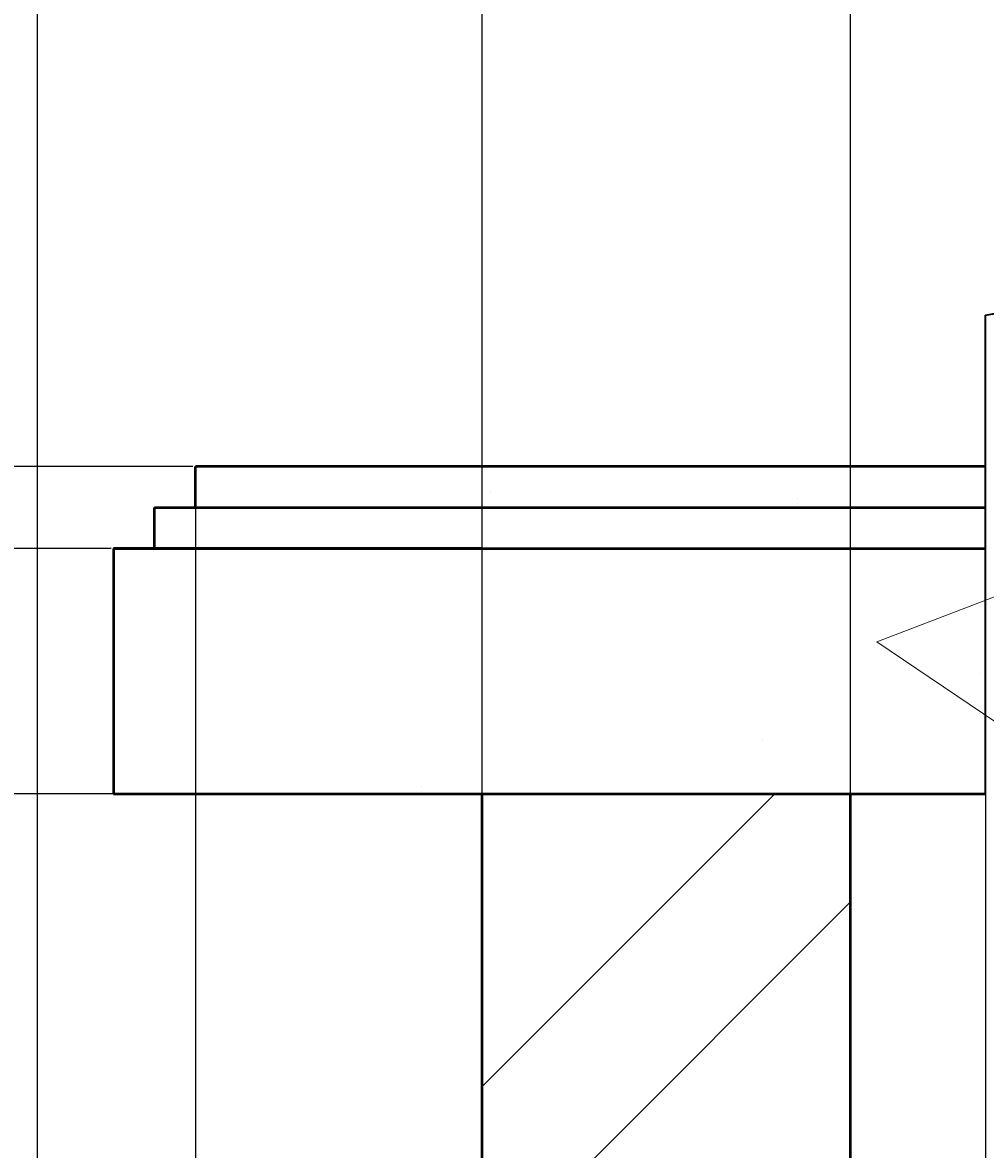
# Model space of a CAD drawing. Units: inches. Extents: x 2812 to 3051, y 1398 to 1659.
# Tile 8 of 65: x 2824 to 2848, y 1473 to 1501. Entities that reach past the tile are written whole.
import ezdxf

# ---------------------------------------------------------------- set-up
doc = ezdxf.new("R2010")
doc.units = ezdxf.units.IN
for name, color, linetype, lineweight in [('A-ANNO-DIMS', 2, 'Continuous', 18), ('P-SANR-PIPE', 4, 'Continuous', 35), ('S-CONC', 7, 'Continuous', 50), ('S-CONC-PATT', 8, 'Continuous', 18)]:
    doc.layers.add(name, color=color, linetype=linetype, lineweight=lineweight)
doc.styles.get("Standard").update_dxf_attribs({"font": 'arial.ttf'})
doc.dimstyles.get("Standard").update_dxf_attribs({"dimtxt": 0.18, "dimasz": 0.18, "dimexe": 0.18, "dimexo": 0.0625, "dimgap": 0.09, "dimtad": 0, "dimtih": 1, "dimtoh": 1, "dimdec": 4, "dimzin": 0, "dimdsep": 46, "dimtxsty": 'Standard', "dimcen": 0.09, "dimadec": 0, "dimazin": 0, "dimtfac": 1, "dimtdec": 4, "dimtofl": 0, "dimtmove": 0, "dimatfit": 3, "dimfxl": 1, "dimtolj": 1, "dimtzin": 0, "dimarcsym": 0})

# ---------------------------------------------------------------- blocks, each defined once
blk = doc.blocks.new('*D27')
at = {"layer": 'A-ANNO-DIMS', "color": 0, "lineweight": -2, "transparency": 16777216}
for p, q in [((2824.521, 1594.167), (2824.521, 1397.505)), ((2835.385, 1550.757), (2835.385, 1397.505)), ((2824.701, 1397.685), (2829.498, 1397.685)), ((2835.205, 1397.685), (2830.408, 1397.685))]:
    blk.add_line(p, q, dxfattribs=at)
at = {"layer": 'A-ANNO-DIMS', "color": 0, "transparency": 16777216}
for points in [[(2824.701, 1397.715), (2824.701, 1397.655), (2824.521, 1397.685)], [(2835.205, 1397.715), (2835.205, 1397.655), (2835.385, 1397.685)]]:
    blk.add_solid(points, dxfattribs=at)
at = {"layer": 'Defpoints', "color": 0, "transparency": 16777216}
for p in [(2824.521, 1594.23), (2835.385, 1550.82), (2835.385, 1397.685)]:
    blk.add_point(p, dxfattribs=at)
at = {"layer": 'A-ANNO-DIMS', "color": 0, "transparency": 16777216, "insert": (2829.953, 1397.685), "char_height": 0.18, "attachment_point": 5}
blk.add_mtext('\\A1;10.863', dxfattribs=at)
blk = doc.blocks.new('*D28')
at = {"layer": 'A-ANNO-DIMS', "color": 0, "lineweight": -2, "transparency": 16777216}
for p, q in [((2851.646, 1598.667), (2851.646, 1397.505)), ((2844.385, 1559.757), (2844.385, 1397.505)), ((2844.565, 1397.685), (2847.64, 1397.685)), ((2851.466, 1397.685), (2848.391, 1397.685))]:
    blk.add_line(p, q, dxfattribs=at)
at = {"layer": 'A-ANNO-DIMS', "color": 0, "transparency": 16777216}
for points in [[(2844.565, 1397.715), (2844.565, 1397.655), (2844.385, 1397.685)], [(2851.466, 1397.715), (2851.466, 1397.655), (2851.646, 1397.685)]]:
    blk.add_solid(points, dxfattribs=at)
at = {"layer": 'Defpoints', "color": 0, "transparency": 16777216}
for p in [(2851.646, 1598.73), (2844.385, 1559.82), (2851.646, 1397.685)]:
    blk.add_point(p, dxfattribs=at)
at = {"layer": 'A-ANNO-DIMS', "color": 0, "transparency": 16777216, "insert": (2848.016, 1397.685), "char_height": 0.18, "attachment_point": 5}
blk.add_mtext('\\A1;7.261', dxfattribs=at)
blk = doc.blocks.new('*D41')
at = {"layer": 'A-ANNO-DIMS', "color": 0, "lineweight": -2, "transparency": 16777216}
for p, q in [((2828.385, 1489.973), (2828.385, 1397.505)), ((2826.385, 1409.973), (2826.385, 1397.505)), ((2826.565, 1397.685), (2827.235, 1397.685)), ((2828.205, 1397.685), (2827.535, 1397.685))]:
    blk.add_line(p, q, dxfattribs=at)
at = {"layer": 'A-ANNO-DIMS', "color": 0, "transparency": 16777216}
for points in [[(2826.565, 1397.715), (2826.565, 1397.655), (2826.385, 1397.685)], [(2828.205, 1397.715), (2828.205, 1397.655), (2828.385, 1397.685)]]:
    blk.add_solid(points, dxfattribs=at)
at = {"layer": 'Defpoints', "color": 0, "transparency": 16777216}
for p in [(2828.385, 1490.035), (2826.385, 1410.035), (2828.385, 1397.685)]:
    blk.add_point(p, dxfattribs=at)
at = {"layer": 'A-ANNO-DIMS', "color": 0, "transparency": 16777216, "insert": (2827.385, 1397.685), "char_height": 0.18, "attachment_point": 5}
blk.add_mtext('\\A1;2', dxfattribs=at)
blk = doc.blocks.new('*D42')
at = {"layer": 'A-ANNO-DIMS', "color": 0, "lineweight": -2, "transparency": 16777216}
for p, q in [((2828.385, 1489.973), (2828.385, 1397.505)), ((2847.686, 1487.973), (2847.686, 1397.505)), ((2828.565, 1397.685), (2837.72, 1397.685)), ((2847.506, 1397.685), (2838.351, 1397.685))]:
    blk.add_line(p, q, dxfattribs=at)
at = {"layer": 'A-ANNO-DIMS', "color": 0, "transparency": 16777216}
for points in [[(2828.565, 1397.715), (2828.565, 1397.655), (2828.385, 1397.685)], [(2847.506, 1397.715), (2847.506, 1397.655), (2847.686, 1397.685)]]:
    blk.add_solid(points, dxfattribs=at)
at = {"layer": 'Defpoints', "color": 0, "transparency": 16777216}
for p in [(2828.385, 1490.035), (2847.686, 1488.035), (2847.686, 1397.685)]:
    blk.add_point(p, dxfattribs=at)
at = {"layer": 'A-ANNO-DIMS', "color": 0, "transparency": 16777216, "insert": (2838.036, 1397.685), "char_height": 0.18, "attachment_point": 5}
blk.add_mtext('\\A1;19.3', dxfattribs=at)
blk = doc.blocks.new('*D51')
at = {"layer": 'A-ANNO-DIMS', "color": 0, "lineweight": -2, "transparency": 16777216}
for p, q in [((2835.322, 1482.035), (2811.806, 1482.035)), ((2811.986, 1481.855), (2811.986, 1472.351)), ((2811.986, 1462.483), (2811.986, 1471.987)), ((2835.322, 1462.303), (2811.806, 1462.303))]:
    blk.add_line(p, q, dxfattribs=at)
at = {"layer": 'A-ANNO-DIMS', "color": 0, "transparency": 16777216}
for points in [[(2811.956, 1481.855), (2812.016, 1481.855), (2811.986, 1482.035)], [(2811.956, 1462.483), (2812.016, 1462.483), (2811.986, 1462.303)]]:
    blk.add_solid(points, dxfattribs=at)
at = {"layer": 'Defpoints', "color": 0, "transparency": 16777216}
for p in [(2811.986, 1482.035), (2835.385, 1482.035), (2835.385, 1462.303)]:
    blk.add_point(p, dxfattribs=at)
at = {"layer": 'A-ANNO-DIMS', "color": 0, "transparency": 16777216, "insert": (2811.986, 1472.169), "char_height": 0.18, "attachment_point": 5}
blk.add_mtext('\\A1;19.733', dxfattribs=at)
blk = doc.blocks.new('*D52')
at = {"layer": 'A-ANNO-DIMS', "color": 0, "lineweight": -2, "transparency": 16777216}
for p, q in [((2826.322, 1488.035), (2811.806, 1488.035)), ((2811.986, 1487.855), (2811.986, 1485.217)), ((2811.986, 1482.215), (2811.986, 1484.853)), ((2826.322, 1482.035), (2811.806, 1482.035))]:
    blk.add_line(p, q, dxfattribs=at)
at = {"layer": 'A-ANNO-DIMS', "color": 0, "transparency": 16777216}
for points in [[(2811.956, 1487.855), (2812.016, 1487.855), (2811.986, 1488.035)], [(2811.956, 1482.215), (2812.016, 1482.215), (2811.986, 1482.035)]]:
    blk.add_solid(points, dxfattribs=at)
at = {"layer": 'Defpoints', "color": 0, "transparency": 16777216}
for p in [(2811.986, 1488.035), (2826.385, 1488.035), (2826.385, 1482.035)]:
    blk.add_point(p, dxfattribs=at)
at = {"layer": 'A-ANNO-DIMS', "color": 0, "transparency": 16777216, "insert": (2811.986, 1485.035), "char_height": 0.18, "attachment_point": 5}
blk.add_mtext('\\A1;6', dxfattribs=at)
blk = doc.blocks.new('*D53')
at = {"layer": 'A-ANNO-DIMS', "color": 0, "lineweight": -2, "transparency": 16777216}
for p, q in [((2828.322, 1490.035), (2811.806, 1490.035)), ((2811.986, 1489.855), (2811.986, 1489.216)), ((2811.986, 1488.215), (2811.986, 1488.855)), ((2826.322, 1488.035), (2811.806, 1488.035))]:
    blk.add_line(p, q, dxfattribs=at)
at = {"layer": 'A-ANNO-DIMS', "color": 0, "transparency": 16777216}
for points in [[(2811.956, 1489.855), (2812.016, 1489.855), (2811.986, 1490.035)], [(2811.956, 1488.215), (2812.016, 1488.215), (2811.986, 1488.035)]]:
    blk.add_solid(points, dxfattribs=at)
at = {"layer": 'Defpoints', "color": 0, "transparency": 16777216}
for p in [(2811.986, 1490.035), (2828.385, 1490.035), (2826.385, 1488.035)]:
    blk.add_point(p, dxfattribs=at)
at = {"layer": 'A-ANNO-DIMS', "color": 0, "transparency": 16777216, "insert": (2811.986, 1489.035), "char_height": 0.18, "attachment_point": 5}
blk.add_mtext('\\A1;2', dxfattribs=at)

msp = doc.modelspace()

# ---------------------------------------------------------------- hatches: boundary and pattern name
at = {"layer": 'S-CONC-PATT'}
h = msp.add_hatch(dxfattribs=at)
h.set_pattern_fill('ANSI32', color=256)
h.paths.add_polyline_path([(3027.3849, 1646.82), (2835.3849, 1646.82), (2835.3849, 1603.2296), (2844.3849, 1603.2296), (2844.3849, 1637.82), (3018.3849, 1637.82), (3018.3849, 1602.5441), (3027.3849, 1602.5441)])
h.paths.add_polyline_path([(2844.3849, 1594.2296), (2835.3849, 1594.2296), (2835.3849, 1550.82), (3027.3849, 1550.82), (3027.3849, 1593.5441), (3018.3849, 1593.5441), (3018.3849, 1559.82), (2844.3849, 1559.82)])
h.paths.add_polyline_path([(2844.3849, 1482.0354), (2835.3849, 1482.0354), (2835.3849, 1463.4959), (2844.3849, 1463.4959)])
h.paths.add_polyline_path([(2844.3849, 1461.4959), (2835.3849, 1461.4959), (2835.3849, 1416.0354), (2844.3849, 1416.0354)])
h.paths.add_polyline_path([(3027.3849, 1482.0354), (3018.3849, 1482.0354), (3018.3849, 1463.2854), (3027.3849, 1463.2854)])
h.paths.add_polyline_path([(3027.3849, 1461.2854), (3018.3849, 1461.2854), (3018.3849, 1416.0354), (3027.3849, 1416.0354)])
h.paths.add_polyline_path([(2961.3849, 1448.4738), (2952.3849, 1448.4738), (2952.3849, 1416.0354), (2961.3849, 1416.0354)])
h.paths.add_polyline_path([(2961.3849, 1462.3026), (2952.3849, 1462.3026), (2952.3849, 1450.4738), (2961.3849, 1450.4738)])
h.paths.add_polyline_path([(2961.3849, 1472.0354), (2952.3849, 1472.0354), (2952.3849, 1462.3026), (2961.3849, 1462.3026)])
h = msp.add_hatch(dxfattribs=at)
h.set_pattern_fill('AR-SAND', color=256, scale=0.3)
h.paths.add_polyline_path([(3036.3849, 1416.0354), (3027.3849, 1416.0354), (2826.3849, 1416.0354), (2826.3849, 1410.0354), (2835.3849, 1410.0354), (3036.3849, 1410.0354)])
h.paths.add_polyline_path([(2970.3849, 1488.0354), (2969.3849, 1488.0354), (2941.3849, 1488.0354), (2941.3849, 1482.0354), (2970.3849, 1482.0354)])
h.paths.add_polyline_path([(3036.3849, 1488.0354), (3035.3849, 1488.0354), (3006.3849, 1488.0354), (3006.3849, 1482.0354), (3027.3849, 1482.0354), (3036.3849, 1482.0354)])
h.paths.add_polyline_path([(3034.3849, 1490.0354), (3008.3849, 1490.0354), (3008.3849, 1489.0354), (3034.3849, 1489.0354)])
h.paths.add_polyline_path([(3035.3849, 1489.0354), (3034.3849, 1489.0354), (3007.3849, 1489.0354), (3007.3849, 1488.0354), (3035.3849, 1488.0354)])
h.paths.add_polyline_path([(2968.3849, 1490.0354), (2943.3849, 1490.0354), (2943.3849, 1489.0354), (2968.3849, 1489.0354)])
h.paths.add_polyline_path([(2969.3849, 1489.0354), (2968.3849, 1489.0354), (2942.3849, 1489.0354), (2942.3849, 1488.0354), (2969.3849, 1488.0354)])
h.paths.add_polyline_path([(2896.3849, 1488.0354), (2826.3849, 1488.0354), (2826.3849, 1482.0354), (2896.3849, 1482.0354)])
h.paths.add_polyline_path([(2895.3849, 1489.0354), (2894.3849, 1489.0354), (2827.3849, 1489.0354), (2827.3849, 1488.0354), (2895.3849, 1488.0354)])
h.paths.add_polyline_path([(2894.3849, 1490.0354), (2828.3849, 1490.0354), (2828.3849, 1489.0354), (2894.3849, 1489.0354)])
h = msp.add_hatch(dxfattribs=at)
h.set_pattern_fill('AR-CONC', color=256, scale=0.3)
h.paths.add_polyline_path([(2896.3849, 1488.0354), (2826.3849, 1488.0354), (2826.3849, 1482.0354), (2896.3849, 1482.0354)])
h.paths.add_polyline_path([(2970.3849, 1488.0354), (2941.3849, 1488.0354), (2941.3849, 1482.0354), (2970.3849, 1482.0354)])
h.paths.add_polyline_path([(2968.3849, 1490.0354), (2943.3849, 1490.0354), (2943.3849, 1489.0354), (2968.3849, 1489.0354)])
h.paths.add_polyline_path([(2969.3849, 1489.0354), (2968.3849, 1489.0354), (2943.3849, 1489.0354), (2942.3849, 1489.0354), (2942.3849, 1488.0354), (2969.3849, 1488.0354)])
h.paths.add_polyline_path([(3036.3849, 1488.0354), (3035.3849, 1488.0354), (3006.3849, 1488.0354), (3006.3849, 1482.0354), (3027.3849, 1482.0354), (3036.3849, 1482.0354)])
h.paths.add_polyline_path([(3035.3849, 1489.0354), (3034.3849, 1489.0354), (3007.3849, 1489.0354), (3007.3849, 1488.0354), (3035.3849, 1488.0354)])
h.paths.add_polyline_path([(3034.3849, 1490.0354), (3008.3849, 1490.0354), (3008.3849, 1489.0354), (3034.3849, 1489.0354)])
h.paths.add_polyline_path([(2895.3849, 1489.0354), (2894.3849, 1489.0354), (2827.3849, 1489.0354), (2827.3849, 1488.0354), (2895.3849, 1488.0354)])
h.paths.add_polyline_path([(2894.3849, 1490.0354), (2828.3849, 1490.0354), (2828.3849, 1489.0354), (2894.3849, 1489.0354)])

# ---------------------------------------------------------------- linework, layer by layer
at = {"layer": 'P-SANR-PIPE'}
msp.add_line((2847.6863, 1482.0354), (2847.6863, 1493.7383), dxfattribs=at)
msp.add_open_spline([(2847.6863, 1493.7383), (2848.165, 1493.8196), (2849.1224, 1493.9821), (2850.4598, 1493.1692), (2850.7485, 1493.7383)], degree=3, dxfattribs=at)
at = {"layer": 'S-CONC'}
for p, q in [((2828.3849, 1489.0354), (2828.3849, 1490.0354)), ((2847.6863, 1490.0354), (2828.3849, 1490.0354)), ((2827.3849, 1489.0354), (2847.6863, 1489.0354)), ((2827.3849, 1488.0354), (2827.3849, 1489.0354)), ((2827.3849, 1489.0354), (2828.3849, 1489.0354)), ((2826.3849, 1488.0354), (2847.6863, 1488.0354)), ((2835.3849, 1488.0354), (2826.3849, 1488.0354)), ((2826.3849, 1488.0354), (2826.3849, 1482.0354)), ((2826.3849, 1488.0354), (2827.3849, 1488.0354)), ((2826.3849, 1482.0354), (2847.6863, 1482.0354)), ((2835.3849, 1482.0354), (2835.3849, 1416.0354)), ((2835.3849, 1482.0354), (2835.3849, 1416.0354)), ((2844.3849, 1482.0354), (2844.3849, 1416.0354)), ((2844.3849, 1482.0354), (2847.6863, 1482.0354))]:
    msp.add_line(p, q, dxfattribs=at)

# ---------------------------------------------------------------- dimensions: what is measured, and where the dimension line sits
at = {"layer": 'A-ANNO-DIMS'}
for base, p1, p2, override, picture, middle in [((2851.6462, 1397.6854), (2844.3849, 1559.82), (2851.6462, 1598.7296), {"dimdec": 3, "dimlfac": 1, "dimrnd": 0, "dimzin": 0, "dimdsep": 46, "dimlunit": 2}, '*D28', (2848.0156, 1397.6854)), ((2835.384907, 1397.685398), (2824.521409, 1594.229631), (2835.384907, 1550.819971), {"dimdec": 3, "dimlfac": 1, "dimrnd": 0, "dimzin": 0, "dimdsep": 46, "dimlunit": 2}, '*D27', (2829.953158, 1397.685398)), ((2828.3849, 1397.6854), (2826.3849, 1410.0354), (2828.3849, 1490.0354), {"dimdec": 0, "dimlfac": 1, "dimrnd": 0, "dimzin": 0, "dimdsep": 46, "dimlunit": 2}, '*D41', (2827.3849, 1397.6854)), ((2847.6863, 1397.6854), (2828.3849, 1490.0354), (2847.6863, 1488.0354), {"dimdec": 1, "dimlfac": 1, "dimrnd": 0, "dimzin": 0, "dimdsep": 46, "dimlunit": 2}, '*D42', (2838.0356, 1397.6854))]:
    dim = msp.add_linear_dim(base=base, p1=p1, p2=p2, dimstyle='Standard', override=override, dxfattribs=at)
    dim.commit()
    dim.dimension.update_dxf_attribs({"geometry": picture, "text_midpoint": middle})
for base, p1, p2, override, picture, middle in [((2811.9855, 1490.0354), (2826.3849, 1488.0354), (2828.3849, 1490.0354), {"dimdec": 0, "dimlfac": 1, "dimrnd": 0, "dimzin": 0, "dimdsep": 46, "dimlunit": 2}, '*D53', (2811.9855, 1489.0354)), ((2811.9855, 1488.0354), (2826.3849, 1482.0354), (2826.3849, 1488.0354), {"dimdec": 0, "dimlfac": 1, "dimrnd": 0, "dimzin": 0, "dimdsep": 46, "dimlunit": 2}, '*D52', (2811.9855, 1485.0354)), ((2811.9855, 1482.0354), (2835.3849, 1462.3026), (2835.3849, 1482.0354), {"dimdec": 3, "dimlfac": 1, "dimrnd": 0, "dimzin": 0, "dimdsep": 46, "dimlunit": 2}, '*D51', (2811.9855, 1472.169))]:
    dim = msp.add_linear_dim(base=base, p1=p1, p2=p2, angle=90, dimstyle='Standard', override=override, dxfattribs=at)
    dim.commit()
    dim.dimension.update_dxf_attribs({"geometry": picture, "text_midpoint": middle})

doc.saveas('drawing.dxf')
